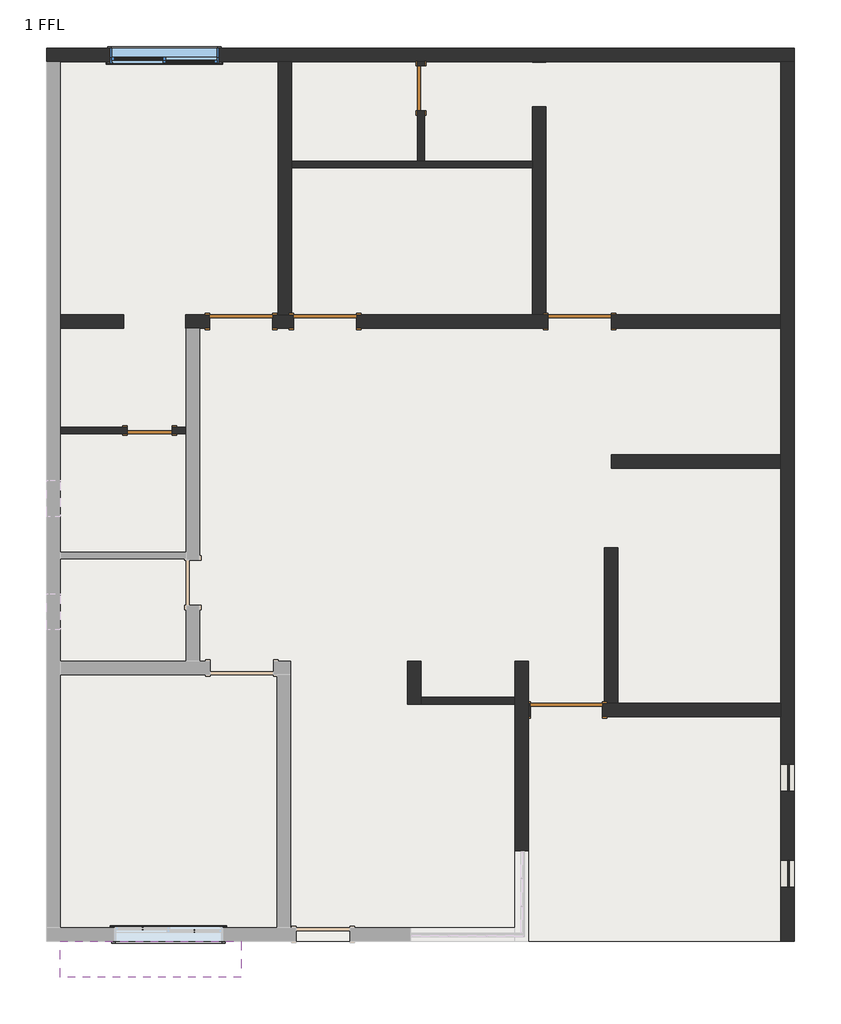
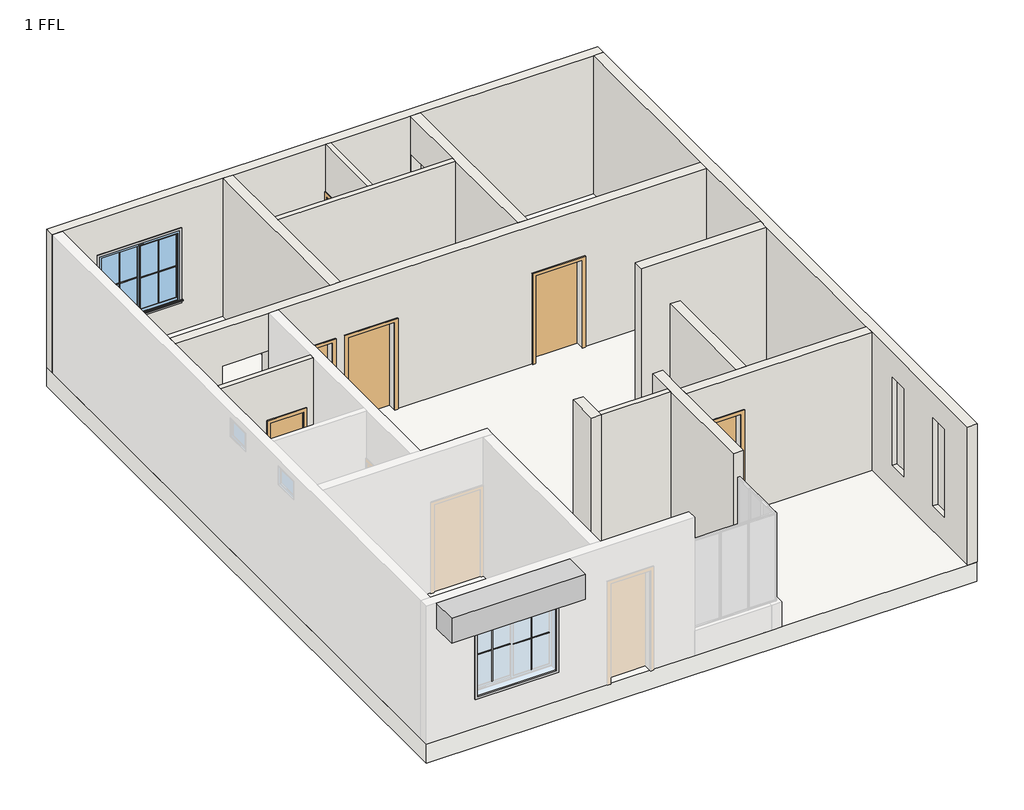
# One storey, part 2 of 2: 16 walls, 9 proxies, 6 doors, 1 slab, 1 window.
"""IFC4 building model written with IfcOpenShell, lengths in millimetres."""

from ifc_helpers import new_model, si_unit, frame, origin, origin_with_axes, place, context, project, spatial, polyline, outline, extrude, faceted_brep, transform, mapped, element, save
from components import generic_models_1_generic_models_1_d7d81bca, muntin_pattern_2x2_muntin_pattern_2x2_52b72501, trim_window_exterior_flat_with_sill_c98b2dec, trim_window_interior_flat_picture_frame_b05ee221, single_flush_9d399b00, single_flush_0848dd25, single_flush_bath_78caadf7, single_flush_bath_214872d5, single_flush_md_e3fbe821, window_sliding_double_89c6b595

model = new_model("IFC4")

# Units and contexts
model_context = context("Model", 3, world=origin())
ifc_project = project(units=[si_unit("LENGTHUNIT", "METRE", prefix="MILLI")], contexts=[model_context])

# Site, building, storey
site = spatial("IfcSite", under=ifc_project)
building = spatial("IfcBuilding", under=site)
storey = spatial("IfcBuildingStorey", under=building, Name="1 FFL", Elevation=0.0)

# Proxies
placement = place(None, origin())
generic_models_1_generic_models_1_shape = generic_models_1_generic_models_1_d7d81bca(model_context)
element("IfcBuildingElementProxy", 1, Name="Generic Models 1 : Generic Models 1", ObjectType="Generic Models 1 : Generic Models 1", at=placement, inside=storey, context=model_context, shape_type="MappedRepresentation", body=[
    mapped(generic_models_1_generic_models_1_shape, transform((0.0, 0.0, 0.0), x_axis=(1.0, 0.0, 0.0), y_axis=(0.0, 1.0, 0.0), z_axis=(0.0, 0.0, 1.0))),
])
muntin_pattern_2x2_muntin_pattern_2x2_shape = muntin_pattern_2x2_muntin_pattern_2x2_52b72501(model_context)
element("IfcBuildingElementProxy", 2, Name="Muntin Pattern_2x2 : Muntin Pattern_2x2", ObjectType="Muntin Pattern_2x2 : Muntin Pattern_2x2", at=placement, inside=storey, context=model_context, shape_type="MappedRepresentation", body=[
    mapped(muntin_pattern_2x2_muntin_pattern_2x2_shape, transform((-3526.8975579, 6961.5453059, 844.55), x_axis=(-1.0, 0.0, 0.0), y_axis=(0.0, -1.0, 0.0), z_axis=(0.0, 0.0, 1.0))),
])
element("IfcBuildingElementProxy", 3, Name="Muntin Pattern_2x2 : Muntin Pattern_2x2", ObjectType="Muntin Pattern_2x2 : Muntin Pattern_2x2", at=placement, inside=storey, context=model_context, shape_type="MappedRepresentation", body=[
    mapped(muntin_pattern_2x2_muntin_pattern_2x2_shape, transform((-2653.7725579, 6917.0953059, 844.55), x_axis=(-1.0, 0.0, 0.0), y_axis=(0.0, -1.0, 0.0), z_axis=(0.0, 0.0, 1.0))),
])
element("IfcBuildingElementProxy", 4, Name="Muntin Pattern_2x2 : Muntin Pattern_2x2", ObjectType="Muntin Pattern_2x2 : Muntin Pattern_2x2", at=placement, inside=storey, context=model_context, shape_type="MappedRepresentation", body=[
    mapped(muntin_pattern_2x2_muntin_pattern_2x2_shape, transform((-2582.8521564, -7786.433484, 844.55), x_axis=(1.0, 0.0, 0.0), y_axis=(0.0, 1.0, 0.0), z_axis=(0.0, 0.0, 1.0))),
])
element("IfcBuildingElementProxy", 5, Name="Muntin Pattern_2x2 : Muntin Pattern_2x2", ObjectType="Muntin Pattern_2x2 : Muntin Pattern_2x2", at=placement, inside=storey, context=model_context, shape_type="MappedRepresentation", body=[
    mapped(muntin_pattern_2x2_muntin_pattern_2x2_shape, transform((-3455.9771564, -7741.983484, 844.55), x_axis=(1.0, 0.0, 0.0), y_axis=(0.0, 1.0, 0.0), z_axis=(0.0, 0.0, 1.0))),
])
trim_window_exterior_flat_with_sill_shape = trim_window_exterior_flat_with_sill_c98b2dec(model_context)
element("IfcBuildingElementProxy", 6, Name="Trim-Window-Exterior-Flat : with Sill", ObjectType="Trim-Window-Exterior-Flat : with Sill", at=placement, inside=storey, context=model_context, shape_type="MappedRepresentation", body=[
    mapped(trim_window_exterior_flat_with_sill_shape, transform((-3090.3350579, 6907.5703059, 2438.4), x_axis=(1.0, 0.0, 0.0), y_axis=(0.0, 0.0, 1.0), z_axis=(0.0, -1.0, 0.0))),
])
element("IfcBuildingElementProxy", 7, Name="Trim-Window-Exterior-Flat : with Sill", ObjectType="Trim-Window-Exterior-Flat : with Sill", at=placement, inside=storey, context=model_context, shape_type="MappedRepresentation", body=[
    mapped(trim_window_exterior_flat_with_sill_shape, transform((-3019.4146564, -7732.458484, 2438.4), x_axis=(-1.0, 0.0, 0.0), y_axis=(0.0, 0.0, 1.0), z_axis=(0.0, 1.0, 0.0))),
])
trim_window_interior_flat_picture_frame_shape = trim_window_interior_flat_picture_frame_b05ee221(model_context)
element("IfcBuildingElementProxy", 8, Name="Trim-Window-Interior-Flat : Picture Frame", ObjectType="Trim-Window-Interior-Flat : Picture Frame", at=placement, inside=storey, context=model_context, shape_type="MappedRepresentation", body=[
    mapped(trim_window_interior_flat_picture_frame_shape, transform((-3090.3350579, 7136.1703059, 2438.4), x_axis=(-1.0, 0.0, 0.0), y_axis=(0.0, 0.0, 1.0), z_axis=(0.0, 1.0, 0.0))),
])
element("IfcBuildingElementProxy", 9, Name="Trim-Window-Interior-Flat : Picture Frame", ObjectType="Trim-Window-Interior-Flat : Picture Frame", at=placement, inside=storey, context=model_context, shape_type="MappedRepresentation", body=[
    mapped(trim_window_interior_flat_picture_frame_shape, transform((-3019.4146564, -7961.058484, 2438.4), x_axis=(1.0, 0.0, 0.0), y_axis=(0.0, 0.0, 1.0), z_axis=(0.0, -1.0, 0.0))),
])

# Doors
single_flush_shape = single_flush_9d399b00(model_context)
element("IfcDoor", 10, ObjectType="Single-Flush", at=placement, inside=storey, context=model_context, shape_type="MappedRepresentation", body=[
    mapped(single_flush_shape, transform((-1792.7942549, 2520.6534118, 0.0), x_axis=(1.0, 0.0, 0.0), y_axis=(0.0, 1.0, 0.0), z_axis=(0.0, 0.0, 1.0))),
])
single_flush_2_shape = single_flush_0848dd25(model_context)
element("IfcDoor", 11, ObjectType="Single-Flush", at=placement, inside=storey, context=model_context, shape_type="MappedRepresentation", body=[
    mapped(single_flush_2_shape, transform((3934.9057451, 2520.6534118, 0.0), x_axis=(-1.0, 0.0, 0.0), y_axis=(0.0, -1.0, 0.0), z_axis=(0.0, 0.0, 1.0))),
])
element("IfcDoor", 12, ObjectType="Single-Flush", at=placement, inside=storey, context=model_context, shape_type="MappedRepresentation", body=[
    mapped(single_flush_2_shape, transform((-370.3942549, 2520.6534118, 0.0), x_axis=(-1.0, 0.0, 0.0), y_axis=(0.0, -1.0, 0.0), z_axis=(0.0, 0.0, 1.0))),
])
single_flush_bath_shape = single_flush_bath_78caadf7(model_context)
element("IfcDoor", 13, ObjectType="Single-Flush : BATH", at=placement, inside=storey, context=model_context, shape_type="MappedRepresentation", body=[
    mapped(single_flush_bath_shape, transform((-3342.1942549, 676.0952215, 0.0), x_axis=(1.0, 0.0, 0.0), y_axis=(0.0, 1.0, 0.0), z_axis=(0.0, 0.0, 1.0))),
])
single_flush_bath_2_shape = single_flush_bath_214872d5(model_context)
element("IfcDoor", 14, ObjectType="Single-Flush : BATH", at=placement, inside=storey, context=model_context, shape_type="MappedRepresentation", body=[
    mapped(single_flush_bath_2_shape, transform((1248.8557451, 6463.0703059, 0.0), x_axis=(0.0, 1.0, 0.0), y_axis=(-1.0, 0.0, 0.0), z_axis=(0.0, 0.0, 1.0))),
])
single_flush_md_shape = single_flush_md_e3fbe821(model_context)
element("IfcDoor", 15, ObjectType="Single-Flush : MD", at=placement, inside=storey, context=model_context, shape_type="MappedRepresentation", body=[
    mapped(single_flush_md_shape, transform((3712.6557451, -4052.5296941, 0.0), x_axis=(1.0, 0.0, 0.0), y_axis=(0.0, 1.0, 0.0), z_axis=(0.0, 0.0, 1.0))),
])

# Slab
element("IfcSlab", 16, ObjectType="6\"", at=placement, inside=storey, context=model_context, shape_type="SweptSolid", body=[
    extrude(outline(polyline([(7553.0590234, 7136.1703059), (7553.0590234, -7961.058484), (-5084.2350579, -7961.058484), (-5084.2350579, 7136.1703059), (7553.0590234, 7136.1703059)])), frame((0.0, 0.0, -457.2), z_axis=(0.0, 0.0, 1.0), x_axis=(1.0, 0.0, 0.0)), (0.0, 0.0, 1.0), 457.2),
])

# Walls
element("IfcWall", 17, ObjectType="1\"", at=placement, inside=storey, context=model_context, shape_type="SweptSolid", body=[
    extrude(outline(polyline([(7478.2057451, -6589.458484), (7478.2057451, -7046.658484), (7452.8057451, -7046.658484), (7452.8057451, -6589.458484), (7478.2057451, -6589.458484)])), frame((0.0, 0.0, 609.6), z_axis=(0.0, 0.0, 1.0), x_axis=(1.0, 0.0, 0.0)), (0.0, 0.0, 1.0), 2133.6),
])
element("IfcWall", 18, ObjectType="1\"", at=placement, inside=storey, context=model_context, shape_type="SweptSolid", body=[
    extrude(outline(polyline([(7478.2057451, -4966.9296941), (7478.2057451, -5424.1296941), (7452.8057451, -5424.1296941), (7452.8057451, -4966.9296941), (7478.2057451, -4966.9296941)])), frame((0.0, 0.0, 609.6), z_axis=(0.0, 0.0, 1.0), x_axis=(1.0, 0.0, 0.0)), (0.0, 0.0, 1.0), 2133.6),
])
element("IfcWall", 19, ObjectType="4.5\"", at=placement, inside=storey, context=model_context, shape_type="SweptSolid", body=[
    extrude(outline(polyline([(1248.8557451, -3836.6296941), (2842.7057451, -3836.6296941), (2842.7057451, -3950.9296941), (1248.8557451, -3950.9296941), (1248.8557451, -3836.6296941)])), origin_with_axes(), (0.0, 0.0, 1.0), 3352.8),
])
element("IfcWall", 20, ObjectType="4.5\"", at=placement, inside=storey, context=model_context, shape_type="SweptSolid", body=[
    extrude(outline(polyline([(2133.6, -2961.1942549), (0.0, -2961.1942549), (0.0, -2719.8942549), (3352.8, -2719.8942549), (3352.8, -4855.6350579), (0.0, -4855.6350579), (0.0, -3723.1942549), (2133.6, -3723.1942549), (2133.6, -2961.1942549)])), frame((0.0, 618.9452215, 0.0), z_axis=(0.0, 1.0, 0.0), x_axis=(0.0, 0.0, 1.0)), (0.0, 0.0, 1.0), 114.3),
])
element("IfcWall", 21, ObjectType="4.5\"", at=placement, inside=storey, context=model_context, shape_type="Brep", body=[
    faceted_brep([(-941.8942549, 5114.7961615, 0.0), (3134.8057451, 5114.7961615, 0.0), (3134.8057451, 5114.7961615, 3352.8), (-941.8942549, 5114.7961615, 3352.8), (-941.8942549, 5229.0961615, 0.0), (-941.8942549, 5229.0961615, 3352.8), (1191.7057451, 5229.0961615, 3352.8), (1306.0057451, 5229.0961615, 3352.8), (3134.8057451, 5229.0961615, 3352.8), (3134.8057451, 5229.0961615, 0.0), (1306.0057451, 5229.0961615, 0.0), (1191.7057451, 5229.0961615, 0.0)], [[[0, 1, 2, 3]], [[4, 5, 6, 7, 8, 9, 10, 11]], [[1, 0, 4, 11, 10, 9]], [[3, 2, 8, 7, 6, 5]], [[0, 3, 5, 4]], [[2, 1, 9, 8]]]),
])
element("IfcWall", 22, ObjectType="4.5\"", at=placement, inside=storey, context=model_context, shape_type="SweptSolid", body=[
    extrude(outline(polyline([(6907.5703059, 0.0), (6844.0703059, 0.0), (6844.0703059, 2133.6), (6082.0703059, 2133.6), (6082.0703059, 0.0), (5229.0961615, 0.0), (5229.0961615, 3352.8), (6907.5703059, 3352.8), (6907.5703059, 0.0)])), frame((1191.7057451, 0.0, 0.0), z_axis=(1.0, 0.0, 0.0), x_axis=(0.0, 1.0, 0.0)), (0.0, 0.0, 1.0), 114.3),
])
element("IfcWall", 23, ObjectType="9\"", at=placement, inside=storey, context=model_context, shape_type="Brep", body=[
    faceted_brep([(-5084.2350579, 6907.5703059, 0.0), (-4855.6350579, 6907.5703059, 0.0), (-1170.4942549, 6907.5703059, 0.0), (-941.8942549, 6907.5703059, 0.0), (1191.7057451, 6907.5703059, 0.0), (1306.0057451, 6907.5703059, 0.0), (3134.8057451, 6907.5703059, 0.0), (3363.4057451, 6907.5703059, 0.0), (7338.5057451, 6907.5703059, 0.0), (7567.1057451, 6907.5703059, 0.0), (7567.1057451, 6907.5703059, 3352.8), (7338.5057451, 6907.5703059, 3352.8), (3363.4057451, 6907.5703059, 3352.8), (3134.8057451, 6907.5703059, 3352.8), (1306.0057451, 6907.5703059, 3352.8), (1191.7057451, 6907.5703059, 3352.8), (-941.8942549, 6907.5703059, 3352.8), (-1170.4942549, 6907.5703059, 3352.8), (-4855.6350579, 6907.5703059, 3352.8), (-5084.2350579, 6907.5703059, 3352.8), (-4004.7350579, 6907.5703059, 2438.4), (-2175.9350579, 6907.5703059, 2438.4), (-2175.9350579, 6907.5703059, 762.0), (-4004.7350579, 6907.5703059, 762.0), (-5084.2350579, 7136.1703059, 0.0), (-5084.2350579, 7136.1703059, 3352.8), (7567.1057451, 7136.1703059, 3352.8), (7567.1057451, 7136.1703059, 0.0), (-4004.7350579, 7136.1703059, 2438.4), (-4004.7350579, 7136.1703059, 762.0), (-2175.9350579, 7136.1703059, 762.0), (-2175.9350579, 7136.1703059, 2438.4)], [[[0, 1, 2, 3, 4, 5, 6, 7, 8, 9, 10, 11, 12, 13, 14, 15, 16, 17, 18, 19], [20, 21, 22, 23]], [[24, 25, 26, 27], [28, 29, 30, 31]], [[9, 8, 7, 6, 5, 4, 3, 2, 1, 0, 24, 27]], [[19, 18, 17, 16, 15, 14, 13, 12, 11, 10, 26, 25]], [[10, 9, 27, 26]], [[0, 19, 25, 24]], [[29, 28, 20, 23]], [[30, 29, 23, 22]], [[31, 30, 22, 21]], [[28, 31, 21, 20]]]),
])
element("IfcWall", 24, ObjectType="9\"", at=placement, inside=storey, context=model_context, shape_type="Brep", body=[
    faceted_brep([(7338.5057451, 6907.5703059, 0.0), (7338.5057451, 2634.9534118, 0.0), (7338.5057451, 2406.3534118, 0.0), (7338.5057451, 267.4142537, 0.0), (7338.5057451, 38.8142537, 0.0), (7338.5057451, -3938.2296941, 0.0), (7338.5057451, -4166.8296941, 0.0), (7338.5057451, -7961.058484, 0.0), (7338.5057451, -7961.058484, 3352.8), (7338.5057451, -4166.8296941, 3352.8), (7338.5057451, -3938.2296941, 3352.8), (7338.5057451, 38.8142537, 3352.8), (7338.5057451, 267.4142537, 3352.8), (7338.5057451, 2406.3534118, 3352.8), (7338.5057451, 2634.9534118, 3352.8), (7338.5057451, 6907.5703059, 3352.8), (7338.5057451, -5424.1296941, 2743.2), (7338.5057451, -5424.1296941, 609.6), (7338.5057451, -4966.9296941, 609.6), (7338.5057451, -4966.9296941, 2743.2), (7338.5057451, -7046.658484, 2743.2), (7338.5057451, -7046.658484, 609.6), (7338.5057451, -6589.458484, 609.6), (7338.5057451, -6589.458484, 2743.2), (7567.1057451, 6907.5703059, 0.0), (7567.1057451, 6907.5703059, 3352.8), (7567.1057451, -7961.058484, 3352.8), (7567.1057451, -7961.058484, 0.0), (7567.1057451, -5424.1296941, 2743.2), (7567.1057451, -4966.9296941, 2743.2), (7567.1057451, -4966.9296941, 609.6), (7567.1057451, -5424.1296941, 609.6), (7567.1057451, -7046.658484, 2743.2), (7567.1057451, -6589.458484, 2743.2), (7567.1057451, -6589.458484, 609.6), (7567.1057451, -7046.658484, 609.6), (7452.8057451, -5424.1296941, 2743.2), (7478.2057451, -5424.1296941, 2743.2), (7478.2057451, -5424.1296941, 609.6), (7452.8057451, -5424.1296941, 609.6), (7478.2057451, -4966.9296941, 609.6), (7452.8057451, -4966.9296941, 609.6), (7478.2057451, -4966.9296941, 2743.2), (7452.8057451, -4966.9296941, 2743.2), (7452.8057451, -7046.658484, 2743.2), (7478.2057451, -7046.658484, 2743.2), (7478.2057451, -7046.658484, 609.6), (7452.8057451, -7046.658484, 609.6), (7478.2057451, -6589.458484, 609.6), (7452.8057451, -6589.458484, 609.6), (7478.2057451, -6589.458484, 2743.2), (7452.8057451, -6589.458484, 2743.2)], [[[0, 1, 2, 3, 4, 5, 6, 7, 8, 9, 10, 11, 12, 13, 14, 15], [16, 17, 18, 19], [20, 21, 22, 23]], [[24, 25, 26, 27], [28, 29, 30, 31], [32, 33, 34, 35]], [[0, 15, 25, 24]], [[7, 6, 5, 4, 3, 2, 1, 0, 24, 27]], [[8, 7, 27, 26]], [[15, 14, 13, 12, 11, 10, 9, 8, 26, 25]], [[17, 16, 36, 37, 28, 31, 38, 39]], [[18, 17, 39, 38, 31, 30, 40, 41]], [[19, 18, 41, 40, 30, 29, 42, 43]], [[16, 19, 43, 42, 29, 28, 37, 36]], [[21, 20, 44, 45, 32, 35, 46, 47]], [[22, 21, 47, 46, 35, 34, 48, 49]], [[23, 22, 49, 48, 34, 33, 50, 51]], [[20, 23, 51, 50, 33, 32, 45, 44]]]),
])
element("IfcWall", 25, ObjectType="9\"", at=placement, inside=storey, context=model_context, shape_type="Brep", body=[
    faceted_brep([(7338.5057451, -3938.2296941, 0.0), (4582.6057451, -3938.2296941, 0.0), (4354.0057451, -3938.2296941, 0.0), (4322.2557451, -3938.2296941, 0.0), (4322.2557451, -3938.2296941, 2438.4), (3103.0557451, -3938.2296941, 2438.4), (3103.0557451, -3938.2296941, 0.0), (3071.3057451, -3938.2296941, 0.0), (3071.3057451, -3938.2296941, 3352.8), (4354.0057451, -3938.2296941, 3352.8), (4582.6057451, -3938.2296941, 3352.8), (7338.5057451, -3938.2296941, 3352.8), (4322.2557451, -4166.8296941, 2438.4), (4322.2557451, -4166.8296941, 0.0), (7338.5057451, -4166.8296941, 0.0), (7338.5057451, -4166.8296941, 3352.8), (3071.3057451, -4166.8296941, 3352.8), (3071.3057451, -4166.8296941, 0.0), (3103.0557451, -4166.8296941, 0.0), (3103.0557451, -4166.8296941, 2438.4)], [[[0, 1, 2, 3, 4, 5, 6, 7, 8, 9, 10, 11]], [[12, 13, 14, 15, 16, 17, 18, 19]], [[18, 17, 7, 6]], [[14, 13, 3, 2, 1, 0]], [[11, 10, 9, 8, 16, 15]], [[8, 7, 17, 16]], [[4, 3, 13, 12]], [[5, 4, 12, 19]], [[6, 5, 19, 18]], [[0, 11, 15, 14]]]),
])
element("IfcWall", 26, ObjectType="9\"", at=placement, inside=storey, context=model_context, shape_type="Brep", body=[
    faceted_brep([(3071.3057451, -6427.4296941, 3352.8), (3071.3057451, -6427.4296941, 2743.2), (3071.3057451, -6427.4296941, 609.6), (3071.3057451, -6427.4296941, 0.0), (3071.3057451, -4166.8296941, 0.0), (3071.3057451, -3938.2296941, 0.0), (3071.3057451, -3227.0296941, 0.0), (3071.3057451, -3227.0296941, 3352.8), (3071.3057451, -3938.2296941, 3352.8), (3071.3057451, -4166.8296941, 3352.8), (2842.7057451, -6427.4296941, 0.0), (2842.7057451, -6427.4296941, 609.6), (2842.7057451, -6427.4296941, 2743.2), (2842.7057451, -6427.4296941, 3352.8), (2842.7057451, -3950.9296941, 3352.8), (2842.7057451, -3836.6296941, 3352.8), (2842.7057451, -3227.0296941, 3352.8), (2842.7057451, -3227.0296941, 0.0), (2842.7057451, -3836.6296941, 0.0), (2842.7057451, -3950.9296941, 0.0)], [[[0, 1, 2, 3, 4, 5, 6, 7, 8, 9]], [[10, 11, 12, 13, 14, 15, 16, 17, 18, 19]], [[6, 5, 4, 3, 10, 19, 18, 17]], [[7, 6, 17, 16]], [[0, 9, 8, 7, 16, 15, 14, 13]], [[0, 13, 12, 11, 10, 3, 2, 1]]]),
])
element("IfcWall", 27, ObjectType="9\"", at=placement, inside=storey, context=model_context, shape_type="Brep", body=[
    faceted_brep([(-1259.3942549, 2406.3534118, 0.0), (-903.7942549, 2406.3534118, 0.0), (-903.7942549, 2406.3534118, 2133.6), (163.0057451, 2406.3534118, 2133.6), (163.0057451, 2406.3534118, 0.0), (3401.5057451, 2406.3534118, 0.0), (3401.5057451, 2406.3534118, 2133.6), (4468.3057451, 2406.3534118, 2133.6), (4468.3057451, 2406.3534118, 0.0), (7338.5057451, 2406.3534118, 0.0), (7338.5057451, 2406.3534118, 3352.8), (-2491.2942549, 2406.3534118, 3352.8), (-2719.8942549, 2406.3534118, 3352.8), (-4855.6350579, 2406.3534118, 3352.8), (-4855.6350579, 2406.3534118, 0.0), (-3782.6504177, 2406.3534118, 0.0), (-3782.6504177, 2406.3534118, 2438.4), (-2730.6641269, 2406.3534118, 2438.4), (-2730.6641269, 2406.3534118, 0.0), (-2719.8942549, 2406.3534118, 0.0), (-2491.2942549, 2406.3534118, 0.0), (-2326.1942549, 2406.3534118, 0.0), (-2326.1942549, 2406.3534118, 2133.6), (-1259.3942549, 2406.3534118, 2133.6), (-903.7942549, 2634.9534118, 2133.6), (-903.7942549, 2634.9534118, 0.0), (-941.8942549, 2634.9534118, 0.0), (-1170.4942549, 2634.9534118, 0.0), (-1259.3942549, 2634.9534118, 0.0), (-1259.3942549, 2634.9534118, 2133.6), (-2326.1942549, 2634.9534118, 2133.6), (-2326.1942549, 2634.9534118, 0.0), (-2730.6641269, 2634.9534118, 0.0), (-2730.6641269, 2634.9534118, 2438.4), (-3782.6504177, 2634.9534118, 2438.4), (-3782.6504177, 2634.9534118, 0.0), (-4855.6350579, 2634.9534118, 0.0), (-4855.6350579, 2634.9534118, 3352.8), (-1170.4942549, 2634.9534118, 3352.8), (-941.8942549, 2634.9534118, 3352.8), (3134.8057451, 2634.9534118, 3352.8), (3363.4057451, 2634.9534118, 3352.8), (7338.5057451, 2634.9534118, 3352.8), (7338.5057451, 2634.9534118, 0.0), (4468.3057451, 2634.9534118, 0.0), (4468.3057451, 2634.9534118, 2133.6), (3401.5057451, 2634.9534118, 2133.6), (3401.5057451, 2634.9534118, 0.0), (3363.4057451, 2634.9534118, 0.0), (3134.8057451, 2634.9534118, 0.0), (163.0057451, 2634.9534118, 0.0), (163.0057451, 2634.9534118, 2133.6)], [[[0, 1, 2, 3, 4, 5, 6, 7, 8, 9, 10, 11, 12, 13, 14, 15, 16, 17, 18, 19, 20, 21, 22, 23]], [[24, 25, 26, 27, 28, 29, 30, 31, 32, 33, 34, 35, 36, 37, 38, 39, 40, 41, 42, 43, 44, 45, 46, 47, 48, 49, 50, 51]], [[14, 36, 35, 15]], [[44, 43, 9, 8]], [[21, 20, 19, 18, 32, 31]], [[50, 49, 48, 47, 5, 4]], [[28, 27, 26, 25, 1, 0]], [[13, 12, 11, 10, 42, 41, 40, 39, 38, 37]], [[14, 13, 37, 36]], [[10, 9, 43, 42]], [[29, 28, 0, 23]], [[30, 29, 23, 22]], [[31, 30, 22, 21]], [[6, 5, 47, 46]], [[7, 6, 46, 45]], [[8, 7, 45, 44]], [[16, 34, 33, 17]], [[34, 16, 15, 35]], [[17, 33, 32, 18]], [[2, 1, 25, 24]], [[3, 2, 24, 51]], [[4, 3, 51, 50]]]),
])
element("IfcWall", 28, ObjectType="9\"", at=placement, inside=storey, context=model_context, shape_type="Brep", body=[
    faceted_brep([(1020.2557451, -3227.0296941, 0.0), (1020.2557451, -3950.9296941, 0.0), (1020.2557451, -3950.9296941, 3352.8), (1020.2557451, -3227.0296941, 3352.8), (1248.8557451, -3227.0296941, 0.0), (1248.8557451, -3227.0296941, 3352.8), (1248.8557451, -3836.6296941, 3352.8), (1248.8557451, -3950.9296941, 3352.8), (1248.8557451, -3950.9296941, 0.0), (1248.8557451, -3836.6296941, 0.0)], [[[0, 1, 2, 3]], [[4, 5, 6, 7, 8, 9]], [[1, 0, 4, 9, 8]], [[3, 2, 7, 6, 5]], [[0, 3, 5, 4]], [[2, 1, 8, 7]]]),
])
element("IfcWall", 29, ObjectType="9\"", at=placement, inside=storey, context=model_context, shape_type="SweptSolid", body=[
    extrude(outline(polyline([(4582.6057451, -1309.3296941), (4582.6057451, -3938.2296941), (4354.0057451, -3938.2296941), (4354.0057451, -1309.3296941), (4582.6057451, -1309.3296941)])), origin_with_axes(), (0.0, 0.0, 1.0), 3352.8),
])
element("IfcWall", 30, ObjectType="9\"", at=placement, inside=storey, context=model_context, shape_type="SweptSolid", body=[
    extrude(outline(polyline([(4468.3057451, 267.4142537), (7338.5057451, 267.4142537), (7338.5057451, 38.8142537), (4468.3057451, 38.8142537), (4468.3057451, 267.4142537)])), origin_with_axes(), (0.0, 0.0, 1.0), 3352.8),
])
element("IfcWall", 31, ObjectType="9\"", at=placement, inside=storey, context=model_context, shape_type="Brep", body=[
    faceted_brep([(3363.4057451, 6907.5703059, 0.0), (3363.4057451, 6907.5703059, 3352.8), (3363.4057451, 2634.9534118, 3352.8), (3363.4057451, 2634.9534118, 0.0), (3363.4057451, 6146.7376466, 0.0), (3363.4057451, 6146.7376466, 2438.4), (3363.4057451, 6899.5176916, 2438.4), (3363.4057451, 6899.5176916, 0.0), (3134.8057451, 6907.5703059, 3352.8), (3134.8057451, 6907.5703059, 0.0), (3134.8057451, 6899.5176916, 0.0), (3134.8057451, 6899.5176916, 2438.4), (3134.8057451, 6146.7376466, 2438.4), (3134.8057451, 6146.7376466, 0.0), (3134.8057451, 5229.0961615, 0.0), (3134.8057451, 5114.7961615, 0.0), (3134.8057451, 2634.9534118, 0.0), (3134.8057451, 2634.9534118, 3352.8), (3134.8057451, 5114.7961615, 3352.8), (3134.8057451, 5229.0961615, 3352.8)], [[[0, 1, 2, 3, 4, 5, 6, 7]], [[8, 9, 10, 11, 12, 13, 14, 15, 16, 17, 18, 19]], [[3, 16, 15, 14, 13, 4]], [[9, 0, 7, 10]], [[2, 1, 8, 19, 18, 17]], [[3, 2, 17, 16]], [[1, 0, 9, 8]], [[5, 12, 11, 6]], [[12, 5, 4, 13]], [[6, 11, 10, 7]]]),
])
element("IfcWall", 32, ObjectType="9\"", at=placement, inside=storey, context=model_context, shape_type="Brep", body=[
    faceted_brep([(-941.8942549, 2634.9534118, 0.0), (-941.8942549, 5114.7961615, 0.0), (-941.8942549, 5229.0961615, 0.0), (-941.8942549, 6907.5703059, 0.0), (-941.8942549, 6907.5703059, 3352.8), (-941.8942549, 5229.0961615, 3352.8), (-941.8942549, 5114.7961615, 3352.8), (-941.8942549, 2634.9534118, 3352.8), (-1170.4942549, 2634.9534118, 0.0), (-1170.4942549, 2634.9534118, 3352.8), (-1170.4942549, 6907.5703059, 3352.8), (-1170.4942549, 6907.5703059, 0.0)], [[[0, 1, 2, 3, 4, 5, 6, 7]], [[8, 9, 10, 11]], [[3, 2, 1, 0, 8, 11]], [[7, 6, 5, 4, 10, 9]], [[0, 7, 9, 8]], [[4, 3, 11, 10]]]),
])

# Window
window_sliding_double_shape = window_sliding_double_89c6b595(model_context)
element("IfcWindow", 33, ObjectType="Window-Sliding-Double", at=placement, inside=storey, context=model_context, shape_type="MappedRepresentation", body=[
    mapped(window_sliding_double_shape, transform((-3090.3350579, 7018.0603059, -152.4), x_axis=(-1.0, 0.0, 0.0), y_axis=(0.0, -1.0, 0.0), z_axis=(0.0, 0.0, 1.0))),
])

save(model, "model.ifc")

# Revit data of these elements
# Type "Muntin Pattern_2x2 : Muntin Pattern_2x2"
#   Width [instance default] = 4' - 0"
#   Thickness = 0' - 0 1/2"
#   Height [instance default] = 4' - 0"
#   Distance = 0' - 0 3/4"
#   Interior Material [instance default] = none
#   Exterior Material [instance default] = none
#   Default Elevation = 0
# Type "Trim-Window-Exterior-Flat : with Sill"
#   Trim Width = 0' - 2 1/4"
#   Trim Thickness_Picture Frame = 0' - 1 1/4"
#   Trim Thickness_with Sill = 0' - 0 3/4"
#   Sill Thickness = 0' - 1 1/4"
#   Opening Width [instance default] = 2' - 0"
#   Opening Height [instance default] = 3' - 0"
#   Default Elevation = 4' - 0"
#   Sill = yes
#   Picture Frame = no
#   Trim Material [instance default] = none
# Type "Trim-Window-Interior-Flat : Picture Frame"
#   Trim Thickness_Picture Frame = 0' - 1 1/4"
#   Trim Width = 0' - 2 1/4"
#   Trim Thickness_with Sill = 0' - 0 3/4"
#   Sill Thickness = 0' - 1 1/4"
#   Opening Width [instance default] = 2' - 0"
#   Opening Height [instance default] = 3' - 0"
#   Default Elevation = 4' - 0"
#   Sill = no
#   Picture Frame = yes
#   Trim Material [instance default] = none
# Type "Single-Flush"
#   Type Mark = "8"
#   Construction Type Id = "MDOOR"
#   Assembly Code = "C1020"
#   Analytic Construction = "Metal"
#   Thickness = 0' - 2"
#   Heat Transfer Coefficient (U) = 0.651978 BTU/(h·ft²·°F)
#   Height = 7' - 0"
#   Trim Projection Ext = 0' - 1"
#   Trim Projection Int = 0' - 1"
#   Trim Width = 0' - 3"
#   Width = 3' - 6"
#   Define Thermal Properties by = 1
#   Door Material = Door - Panel
#   Frame Material = Door - Frame
#   Visual Light Transmittance = 0
#   Solar Heat Gain Coefficient = 0
#   Function = (empty or 0)
#   Wall Closure = (empty or 0)
# Type "Single-Flush : BATH"
#   Type Mark = "9"
#   Construction Type Id = "MDOOR"
#   Assembly Code = "C1020"
#   Analytic Construction = "Metal"
#   Thickness = 0' - 2"
#   Heat Transfer Coefficient (U) = 0.651978 BTU/(h·ft²·°F)
#   Height = 7' - 0"
#   Trim Projection Ext = 0' - 1"
#   Trim Projection Int = 0' - 1"
#   Trim Width = 0' - 3"
#   Width = 2' - 6"
#   Define Thermal Properties by = 1
#   Door Material = Door - Panel
#   Frame Material = Door - Frame
#   Visual Light Transmittance = 0
#   Solar Heat Gain Coefficient = 0
#   Function = (empty or 0)
#   Wall Closure = (empty or 0)
# Type "Single-Flush : MD"
#   Type Mark = "10"
#   Construction Type Id = "MDOOR"
#   Assembly Code = "C1020"
#   Analytic Construction = "Metal"
#   Thickness = 0' - 2"
#   Heat Transfer Coefficient (U) = 0.651978 BTU/(h·ft²·°F)
#   Height = 8' - 0"
#   Trim Projection Ext = 0' - 1"
#   Trim Projection Int = 0' - 1"
#   Trim Width = 0' - 3"
#   Width = 4' - 0"
#   Define Thermal Properties by = 1
#   Door Material = Door - Panel
#   Frame Material = Door - Frame
#   Visual Light Transmittance = 0
#   Solar Heat Gain Coefficient = 0
#   Function = (empty or 0)
#   Wall Closure = (empty or 0)
# Type "6\""
#   Assembly Code = "B1010"
#   Function = 0
#   Layers, outside or top first: 1' - 6" no material (function 1)
# Type "1\""
#   Assembly Code = "B2010"
#   Layers, outside or top first: 0' - 1" no material (function 1)
# Type "4.5\""
#   Assembly Code = "B2010"
#   Layers, outside or top first: 0' - 4 1/2" no material (function 1)
# Type "9\""
#   Assembly Code = "B2010"
#   Layers, outside or top first: 0' - 9" no material (function 1)
# Type "Window-Sliding-Double"
#   Type Mark = "19"
#   Fire Rating = "0.5h"
#   Assembly Code = "B2020100"
#   Analytic Construction = "Double glazing - domestic"
#   Window Inset [instance default] = 0' - 0"
#   Wall Thickness [instance default] = 0' - 6"
#   Visual Light Transmittance = 0.81
#   Thermal Resistance (R) = 1.8146 (h·ft²·°F)/BTU
#   Solar Heat Gain Coefficient = 0.76
#   Muntin Width = 2' - 8 5/8"
#   Muntin Height = 5' - 0 1/4"
#   Interior Wall Closure [instance default] = 0' - 2 3/4"
#   Heat Transfer Coefficient (U) = 0.5511 BTU/(h·ft²·°F)
#   Frame Extension [instance default] = 0' - 0 1/4"
#   Exterior Wall Closure [instance default] = 0' - 1 1/4"
#   Rough Width = 6' - 0 1/2"
#   Rough Height = 5' - 6 1/2"
#   Height = 5' - 6"
#   Extension Jamb [instance default] = 0' - 2 3/4"
#   Default Sill Height = 3' - 0"
#   Width = 6' - 0"
#   Interior Trim Visibility [instance default] = yes
#   Indicator Visibility [instance default] = yes
#   Exterior Trim Visibility [instance default] = yes
#   Muntin Visibility = yes
#   Extension Jamb Visibility [instance default] = yes
#   Muntin Pattern = Muntin Pattern_2x2 : Muntin Pattern_2x2
#   Interior Trim Material = Wood - Stained
#   Interior Trim = Trim-Window-Interior-Flat : Picture Frame
#   Interior Frame Material = Wood - Stained
#   Glass Panel Material = Glass
#   Exterior Trim Material = Clad - White
#   Exterior Trim = Trim-Window-Exterior-Flat : with Sill
#   Exterior Frame Material = Clad - White
#   Wall Closure = (empty or 0)
# Element 1 (IfcBuildingElementProxy, "Generic Models 1 : Generic Models 1")
#   Phase Created = New Construction
# Elements 2, 3, 4, 5 (IfcBuildingElementProxy, "Muntin Pattern_2x2 : Muntin Pattern_2x2")
#   Width = 2' - 8 5/8"
#   Height = 5' - 0 1/4"
#   Interior Material = Wood - Stained
#   Exterior Material = Clad - White
#   Phase Created = New Construction
#   Materials on its faces: "Clad - White", "Wood - Stained"
# Elements 6, 7 (IfcBuildingElementProxy, "Trim-Window-Exterior-Flat : with Sill")
#   Opening Width = 6' - 0"
#   Opening Height = 5' - 6"
#   Trim Material = Clad - White
#   Phase Created = New Construction
#   Materials on its faces: "Clad - White"
# Elements 8, 9 (IfcBuildingElementProxy, "Trim-Window-Interior-Flat : Picture Frame")
#   Opening Width = 6' - 0"
#   Opening Height = 5' - 6"
#   Trim Material = Wood - Stained
#   Phase Created = New Construction
#   Materials on its faces: "Wood - Stained"
# Elements 10, 11, 12 (IfcDoor, "Single-Flush")
#   Phase Created = New Construction
#   Materials on its faces: "Door - Frame", "Door - Panel"
# Elements 13, 14 (IfcDoor, "Single-Flush : BATH")
#   Phase Created = New Construction
#   Materials on its faces: "Door - Frame", "Door - Panel"
# Element 15 (IfcDoor, "Single-Flush : MD")
#   Phase Created = New Construction
#   Materials on its faces: "Door - Frame", "Door - Panel"
# Element 16 (IfcSlab, "6\"")
#   Height Offset From Level = 0' - 0"
#   Phase Created = New Construction
#   Materials on its faces: "Default Floor"
# Elements 17, 18 (IfcWall, "1\"")
#   built-in parameter 1001111 = 2' - 0"
#   Top Offset = 0' - 0"
#   Base Offset = 2' - 0"
#   Unconnected Height = 7' - 0"
#   wall height = 7' - 0"
#   Phase Created = New Construction
#   Base Constraint = 1 FFL
#   Materials on its faces: "Default Wall"
# Elements 19, 20, 21, 22 (IfcWall, "4.5\"")
#   Top Offset = 0' - 0"
#   Base Offset = 0' - 0"
#   wall height = 11' - 0"
#   Phase Created = New Construction
#   Base Constraint = 1 FFL
#   Top Constraint = 2 FIRST FLOOR BASE
#   Materials on its faces: "Default Wall"
# Elements 23, 24, 25, 27, 28, 29, 30, 31, 32 (IfcWall, "9\"")
#   Top Offset = 0' - 0"
#   Base Offset = 0' - 0"
#   wall height = 11' - 0"
#   Phase Created = New Construction
#   Base Constraint = 1 FFL
#   Top Constraint = 2 FIRST FLOOR BASE
#   Materials on its faces: "Default Wall"
# Element 26 (IfcWall, "9\"")
#   Top Offset = 0' - 0"
#   Base Offset = 0' - 0"
#   wall height = 11' - 0"
#   Phase Created = New Construction
#   Base Constraint = 1 FFL
#   Top Constraint = 2 FIRST FLOOR BASE
#   Materials on its faces: "Default Wall", "outer wall"
# Element 33 (IfcWindow, "Window-Sliding-Double")
#   Mark = "1"
#   Window Inset = 0' - 0"
#   Interior Wall Closure = 0' - 2 3/4"
#   Frame Extension = 0' - 0 1/4"
#   Exterior Wall Closure = 0' - 1 1/4"
#   Interior Trim Visibility = yes
#   Indicator Visibility = yes
#   Exterior Trim Visibility = yes
#   Phase Created = New Construction
#   Materials on its faces: "Wood - Stained", "Glass", "Clad - White"
# Materials
#   "Door - Panel": class "Wood", colour RGB 210 159 95, transparency 0, Cost = 0
#   "Door - Frame": colour RGB 118 70 51, transparency 0, Cost = 0
#   "Wood - Stained": class "Wood", colour RGB 224 178 126, transparency 0, Cost = 0
#   "Glass": class "Glass", colour RGB 0 128 192, transparency 0.75, Description = "Soda Lime Glass", Cost = 0
#   "Clad - White": class "Wood", colour RGB 242 242 238, transparency 0, Cost = 0
#   "Default Floor": colour RGB 128 128 128, transparency 0, Cost = 0
#   "Default Wall": colour RGB 128 128 128, transparency 0, Cost = 0
#   "outer wall": class "Generic", colour RGB 85 88 91, transparency 0, Cost = 0
